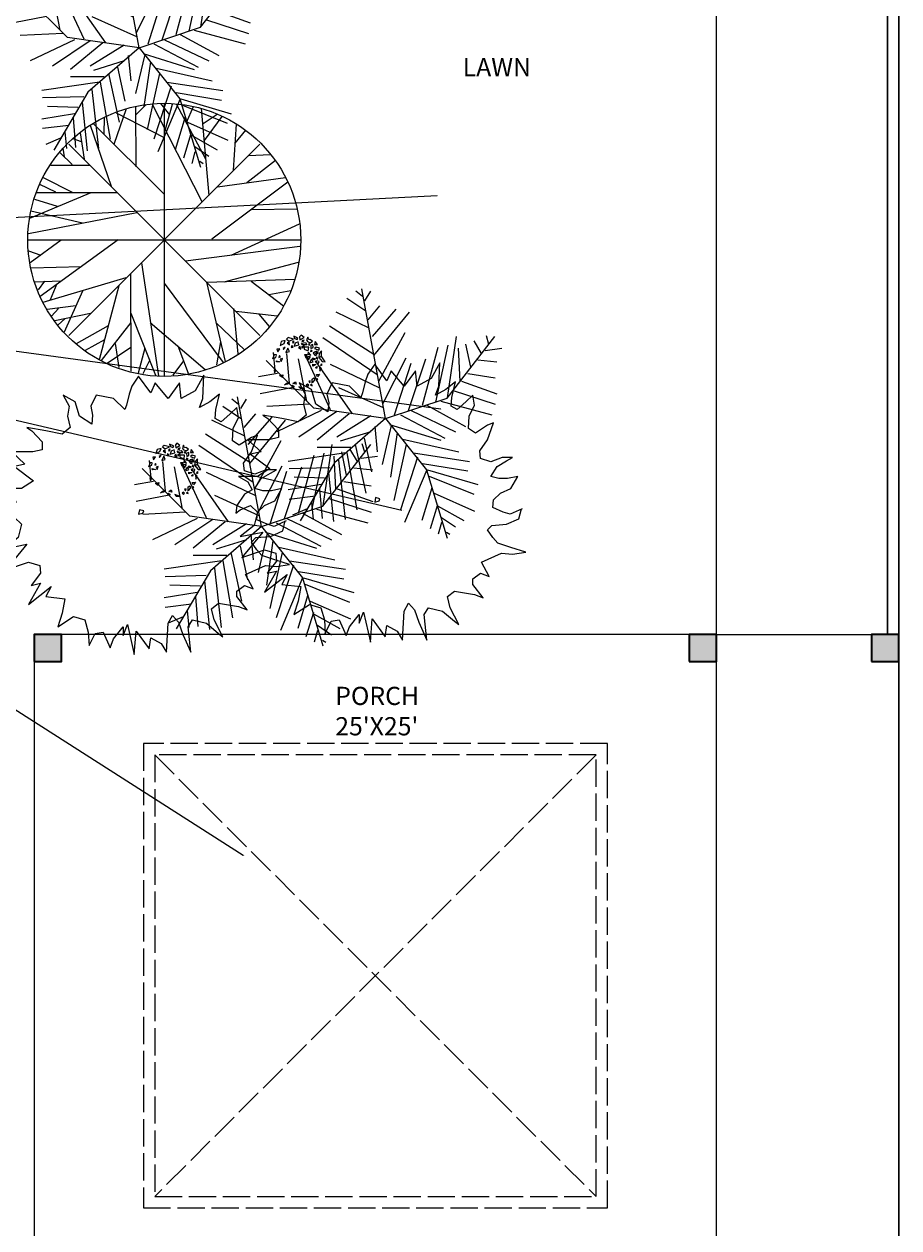
# Model space of a CAD drawing. Units: inches. Extents: x 2330 to 3943, y 1763 to 3461.
# Tile 23 of 40: x 3423 to 3808, y 2300 to 2829. Entities that reach past the tile are written whole.
import ezdxf

# ---------------------------------------------------------------- set-up
doc = ezdxf.new("R2010")
doc.units = ezdxf.units.IN
doc.linetypes.add('ACAD_ISO02W100', pattern=[15, 12, -3])
for name, color, linetype, lineweight in [('A-ANNO-DIMS', 2, 'Continuous', 18), ('A-ANNO-TEXT', 7, 'Continuous', 18), ('A-AREA-IDEN', 7, 'Continuous', 18), ('A-COLS', 7, 'Continuous', 35), ('A-FLOR', 7, 'Continuous', 25), ('A-ROOF-OVHD', 8, 'ACAD_ISO02W100', 18), ('C-PROP', 7, 'Continuous', 30), ('L-PLNT', 94, 'Continuous', 13)]:
    doc.layers.add(name, color=color, linetype=linetype, lineweight=lineweight)
doc.styles.get("Standard").update_dxf_attribs({"font": 'arial.ttf'})
doc.dimstyles.get("Standard").update_dxf_attribs({"dimtxt": 0.18, "dimasz": 0.18, "dimexe": 0.18, "dimexo": 0.0625, "dimgap": 0.09, "dimtad": 0, "dimtih": 1, "dimtoh": 1, "dimdec": 4, "dimzin": 0, "dimdsep": 46, "dimtxsty": 'Standard', "dimcen": 0.09, "dimadec": 0, "dimazin": 0, "dimtfac": 1, "dimtdec": 4, "dimtofl": 0, "dimtmove": 0, "dimatfit": 3, "dimfxl": 1, "dimtolj": 1, "dimtzin": 0, "dimarcsym": 0})

# ---------------------------------------------------------------- blocks, each defined once
blk = doc.blocks.new('*U12')
for p, q in [((-10.186, 53.64), (-13.084, 55.962)), ((0, 0), (-10.5, 57)), ((-9.099, 51.782), (-6.563, 55.962)), ((-8.737, 47.138), (-17.069, 52.711)), ((-7.65, 43.423), (-2.578, 49.46)), ((-5.839, 35.992), (4.667, 48.067)), ((-7.288, 39.707), (-21.778, 46.673)), ((-5.114, 27.632), (10.463, 46.673)), ((-5.114, 28.097), (-24.676, 40.636)), ((-2.941, 16.486), (8.652, 37.85)), ((-3.665, 19.273), (-27.574, 35.527)), ((22.055, 7.198), (27.489, 32.277)), ((27, 9), (48, 36)), ((27.127, 9.056), (31.112, 35.992)), ((35.096, 32.741), (37.27, 22.524)), ((38.719, 34.134), (41.979, 28.561)), ((44.153, 36.456), (45.239, 32.741)), ((-48.585, 21.131), (-49.309, 29.026)), ((-43.513, 28.561), (-42.427, 15.558)), ((-35.544, 28.097), (-24.314, 3.947)), ((-1.129, 6.734), (9.014, 26.704)), ((16.259, 5.805), (23.142, 31.348)), ((31.836, 30.883), (32.561, 16.486)), ((43.791, 29.954), (51.036, 30.883)), ((-31.5, 4.5), (-52.5, 25.5)), ((-38.442, 26.239), (-34.819, 7.663)), ((-14.533, 2.09), (-30.834, 25.31)), ((-24.314, 23.917), (-2.941, 13.7)), ((3.942, 1.625), (11.187, 24.381)), ((10.101, 3.483), (17.708, 26.239)), ((40.53, 25.775), (48.862, 24.846)), ((-47.498, 19.737), (-55.83, 18.344)), ((33.285, 16.486), (48.862, 10.913)), ((36.183, 19.737), (48.137, 17.88)), ((-40.615, 13.7), (-55.105, 10.913)), ((-20.691, 13.7), (-1.129, 4.876)), ((29.662, 12.307), (48.137, 6.269)), ((-33.37, 6.269), (-52.207, 5.34)), ((0, 0), (27, 9)), ((18.07, 5.805), (35.096, -3.483)), ((24.229, 7.663), (46.688, 1.625)), ((-28.299, 3.483), (-47.86, -5.805)), ((-21.416, 3.018), (-38.079, -8.128)), ((0, 0), (-31.5, 4.5)), ((-15.982, 2.09), (-30.11, -9.521)), ((0, 0), (-22.5, -19.5)), ((-6.563, 1.161), (-21.416, -8.128)), ((0, 0), (18, -22.5)), ((6.478, 1.625), (26.04, -8.592)), ((11.187, 3.483), (30.749, -5.805)), ((-4.752, -3.483), (-3.665, -14.629)), ((2.493, -3.019), (-1.491, -20.202)), ((1.769, -2.555), (24.229, -9.521)), ((-6.563, -5.805), (-19.967, -9.985)), ((-9.461, -8.592), (-6.201, -23.453)), ((5.029, -6.27), (2.131, -25.775)), ((7.565, -9.056), (32.198, -14.629)), ((-17.431, -15.094), (-42.789, -18.809)), ((-15.257, -12.772), (-30.11, -12.772)), ((-17.069, -15.094), (-12.721, -40.172)), ((-13.446, -11.378), (-8.737, -32.741)), ((9.014, -11.378), (3.58, -35.992)), ((12.274, -15.094), (36.907, -18.809)), ((-22.5, -19.5), (-37.5, -45)), ((-20.691, -18.345), (-17.793, -44.352)), ((14.085, -16.951), (6.478, -40.172)), ((16.259, -19.738), (36.183, -22.989)), ((-24.314, -21.596), (-42.427, -22.06)), ((-26.849, -26.24), (-40.253, -25.775)), ((-25.038, -23.918), (-22.865, -45.281)), ((18.07, -22.524), (8.289, -45.745)), ((18, -22.5), (27, -52.5)), ((18.433, -22.524), (40.53, -29.026)), ((19.157, -25.311), (38.719, -33.206)), ((-28.299, -29.026), (-42.789, -31.348)), ((-29.023, -30.884), (-27.936, -43.887)), ((20.244, -30.419), (15.897, -44.816)), ((-30.834, -34.135), (-42.427, -35.528)), ((-32.646, -36.921), (-31.921, -44.352)), ((21.331, -32.741), (39.081, -40.636)), ((-34.457, -39.708), (-40.978, -42.494)), ((22.78, -37.85), (19.519, -48.532)), ((22.78, -38.314), (34.372, -44.816)), ((24.591, -45.745), (23.142, -50.854)), ((24.591, -43.423), (30.749, -47.603)), ((26.764, -49.925), (28.213, -50.854))]:
    blk.add_line(p, q)
blk = doc.blocks.new('*U14')
for p, q in [((-12.5388, 54.9406), (-7.9613, 59.4546)), ((-12.3627, 32.1443), (-12.5388, 58.7776)), ((-5.3205, 59.6806), (16.5105, 16.7963)), ((2.426, 54.9406), (-1.4472, 59.9056)), ((0, 59.9996), (0, -60)), ((0.4894, 48.6208), (3.6584, 59.6806)), ((18.2711, 35.5298), (5.419, 59.6806)), ((9.8203, 51.5549), (12.8133, 58.5516)), ((-26.4472, 46.5894), (-26.2712, 53.8116)), ((-22.0458, 42.0753), (-16.5881, 57.6486)), ((-21.1656, 55.8436), (-0.0388, 45.0094)), ((19.6795, 19.5047), (16.3344, 57.6486)), ((17.0387, 51.1035), (23.2006, 55.1666)), ((17.7429, 43.6552), (25.4894, 54.2636)), ((-32.6092, 50.4264), (-23.2782, 23.5674)), ((-31.2008, 51.1035), (-0.2149, 20.1818)), ((31.6513, 50.8778), (30.2429, 30.5643)), ((31.1232, 42.5267), (35.8767, 48.1693)), ((-40.1797, 44.558), (-36.4825, 43.2038)), ((-37.0107, 47.0408), (-35.25, 35.5298)), ((-45.8134, 38.2383), (-40.5318, 33.0471)), ((-43.8768, 36.4326), (-44.405, 40.2696)), ((42, 42), (-42, -42)), ((42, -42), (-42, 42)), ((37.1091, 37.1098), (46.6161, 37.5612)), ((-49.8627, 32.8214), (-32.7853, 32.8214)), ((36.2288, 25.1474), (48.9049, 35.0784)), ((-53.2078, 27.4044), (-40.1797, 20.859)), ((23.3767, 23.3417), (53.3063, 27.4044)), ((-54.7923, 24.4702), (-47.75, 21.0847)), ((54.3626, 25.3731), (20.9119, 0.3198)), ((-32.2571, 20.6333), (-59.1937, 9.348)), ((-57.081, 17.9248), (-47.0458, 14.7649)), ((-56.0247, 20.859), (-20.8134, 20.859)), ((-59.7219, 2.8025), (-12.0106, 12.0565)), ((-58.6656, 12.7336), (-35.9543, 7.5424)), ((38.5175, 13.4107), (58.2359, 13.6364)), ((29.3626, -6.6771), (59.4682, 7.091)), ((-54.6162, -24.7335), (-20.2853, 0.0941)), ((-60, 0), (60, 0)), ((-59.7219, -4.8714), (-54.2641, -6.6771)), ((-45.2853, -0.1316), (-59.0177, -10.0627)), ((9.2922, -9.1598), (59.6443, -2.8401)), ((-10.074, -10.0627), (-2.5036, -59.7178)), ((26.3697, -18.4138), (58.9401, -9.8369)), ((-58.4895, -12.3197), (-36.4825, -11.6426)), ((-14.8275, -15.0282), (-14.6515, -57.6865)), ((-57.081, -18.4138), (-45.2853, -17.9624)), ((-52.6797, -18.188), (-55.4966, -22.0251)), ((-53.2078, -27.442), (-16.7641, -16.6081)), ((-47.2219, -19.3166), (-50.2148, -26.3135)), ((-19.9331, -20.2194), (-28.5599, -52.721)), ((-0.0388, -19.0909), (25.8415, -53.8495)), ((18.6232, -18.6394), (26.7218, -53.3981)), ((18.7992, -18.6394), (57.3556, -17.2853)), ((38.1654, -18.188), (52.426, -29.0219)), ((-35.9543, -22.4765), (-44.0529, -40.5329)), ((45.9119, -24.0564), (55.595, -22.2508)), ((-38.9472, -29.0219), (-51.4472, -30.6018)), ((-46.5177, -30.1504), (-49.5106, -33.536)), ((30.419, -30.1504), (32.3556, -50.0125)), ((31.4753, -31.279), (49.6091, -33.3103)), ((-32.4331, -32.4075), (-48.1021, -35.5674)), ((-43.7008, -34.6645), (-46.6937, -37.373)), ((-14.6515, -36.2445), (-27.6797, -52.9467)), ((-14.6515, -32.1818), (-3.912, -59.4922)), ((-6.2008, -36.2445), (17.919, -57.0094)), ((22.8485, -36.4702), (35.3485, -48.4326)), ((41.5105, -32.6332), (46.088, -38.0501)), ((-24.6867, -37.8244), (-38.7712, -45.7241)), ((-26.2712, -43.9185), (-34.7219, -48.6583)), ((-14.6515, -47.3041), (-25.0388, -54.3009)), ((-21.5177, -45.4984), (-19.9331, -56.1065)), ((-8.4895, -47.5298), (-11.4825, -58.5893)), ((5.9471, -46.6269), (10.5246, -58.5893)), ((24.7852, -44.8213), (23.0246, -54.978)), ((-6.3768, -52.721), (-9.3698, -58.815)), ((8.4119, -53.1724), (3.8344, -59.4922))]:
    blk.add_line(p, q)
blk.add_circle((0, 0), 60)
blk = doc.blocks.new('*U15')
for points in [[(0, 60.64), (-3.051, 56.238), (-4.196, 52.815), (-5.34, 47.925), (-6.103, 45.969), (-11.062, 50.859), (-18.691, 52.326), (-20.98, 47.436), (-20.217, 43.524), (-20.598, 39.611), (-25.939, 43.035), (-27.846, 49.392), (-33.186, 52.326), (-30.516, 47.436), (-31.279, 43.035), (-30.135, 38.144), (-33.568, 35.21), (-40.815, 36.677), (-49.208, 38.144), (-46.919, 36.677), (-42.341, 31.787), (-42.341, 28.364), (-46.537, 27.386), (-55.692, 27.386), (-49.97, 22.006), (-54.548, 21.028), (-46.156, 14.671), (-51.496, 11.248), (-59.888, 11.248), (-55.692, 8.803), (-53.785, 5.38), (-57.218, 3.423), (-60.651, -1.467), (-61.033, -4.89), (-59.125, -3.423), (-54.548, -1.467), (-51.496, -4.401), (-53.022, -10.269), (-59.125, -15.16), (-49.208, -13.204), (-58.362, -24.451), (-48.445, -21.028), (-43.486, -22.495), (-43.104, -25.918), (-47.3, -31.298), (-43.104, -30.32), (-48.445, -39.611), (-38.527, -31.787), (-40.815, -36.188), (-32.423, -37.166), (-33.568, -43.523), (-35.475, -49.392), (-28.609, -44.99), (-23.65, -46.457), (-22.124, -51.837), (-21.743, -57.705), (-19.073, -52.326), (-15.639, -51.837), (-12.588, -58.683), (-11.062, -54.771), (-6.866, -49.392), (-6.866, -53.304), (-4.959, -48.414), (-1.907, -61.617), (-1.144, -51.348), (4.578, -59.172), (5.341, -54.282), (9.918, -56.727), (12.207, -60.639), (12.97, -47.925), (14.877, -44.501), (17.547, -47.436), (19.455, -52.815), (22.888, -60.639), (21.743, -49.392), (23.65, -46.457), (29.754, -47.925), (35.094, -52.326), (37.001, -53.793), (33.187, -46.457), (32.042, -41.567), (35.094, -39.122), (43.868, -40.589), (47.682, -42.056), (43.105, -36.188), (43.105, -33.743), (46.538, -31.298), (50.352, -32.765), (46.919, -26.407), (55.693, -22.495), (60.652, -22.984), (66.374, -22.006), (59.889, -20.05), (54.167, -18.094), (51.878, -15.649), (49.589, -12.225), (51.497, -10.269), (57.981, -9.78), (63.322, -7.335), (64.466, -2.934)], [(64.848, -2.934), (59.507, -5.379), (56.456, -4.401), (51.878, -2.445), (52.26, 0.978), (55.311, 3.912), (59.889, 5.869), (62.94, 11.248), (58.363, 10.27), (54.548, 10.27), (51.115, 11.248), (53.785, 15.649), (57.981, 18.094), (60.652, 19.561), (56.074, 19.561), (51.115, 17.605), (46.538, 19.072), (46.156, 22.496), (49.589, 27.386), (52.26, 34.721), (49.589, 33.743), (44.249, 30.32), (41.197, 32.276), (41.579, 37.655), (43.868, 42.546), (43.105, 46.947), (40.053, 44.013), (36.238, 40.589), (33.568, 42.057), (33.95, 45.969), (35.476, 52.815), (31.28, 49.392), (26.702, 46.947), (28.228, 50.859), (28.609, 61.129), (24.795, 54.282), (18.692, 50.859), (17.929, 57.706), (12.97, 50.859), (7.248, 57.706), (5.341, 53.304), (0, 60.64)]]:
    blk.add_lwpolyline(points)
blk.add_lwpolyline([(0.382, 1.956), (0, 0), (1.907, 0.489), (2.289, 1.467)], close=True)
blk = doc.blocks.new('*U13')
for points in [[(-4.43, 11.05), (-5.18, 10.36), (-3.96, 9.49), (-2.07, 10.36)], [(-2, 11.66), (-1.6, 10.62), (-0.52, 10.1), (-0.18, 10.62), (-0.79, 10.96)], [(1.24, 12), (0.56, 11.31), (0.76, 10.01), (2.52, 11.05)], [(4.14, 11.14), (3.6, 10.01), (4, 9.23), (5.22, 8.71), (6.3, 9.41), (5.08, 10.19), (4.61, 10.01)], [(-8.14, 6.03), (-9.36, 5.95), (-9.02, 4.73)], [(-5.78, 9.75), (-7.54, 9.23), (-8.01, 7.5), (-6.26, 8.45)], [(-5.78, 6.81), (-6.66, 6.21), (-6.52, 5.69)], [(-4.57, 6.38), (-5.45, 4.47), (-3.89, 4.82)], [(-4.84, 8.63), (-3.83, 7.85), (-4.03, 8.97)], [(-2.88, 7.5), (-3.15, 6.64), (-2.27, 6.72)], [(-1.94, 9.49), (-2.48, 8.97), (-2.27, 8.54), (-1.8, 9.06)], [(0.02, 9.06), (-1.33, 8.54), (-1.73, 7.16), (0.29, 7.76)], [(0.76, 7.16), (0.09, 6.46), (1.1, 5.95)], [(1.37, 8.54), (3.13, 8.8), (3.8, 7.85), (1.91, 7.76)], [(2.59, 9.93), (1.84, 9.75), (1.64, 9.23), (2.32, 9.41)], [(1.71, 6.29), (1.71, 7.07), (2.65, 7.5), (2.11, 6.9)], [(2.52, 6.81), (2.52, 5.86), (4.41, 5.17), (4.61, 6.72)], [(4.61, 8.28), (4.54, 7.76), (4.95, 7.59), (4.95, 8.28)], [(5.49, 5.51), (5.42, 4.82), (6.16, 5.08)], [(6.43, 7.94), (5.49, 7.68), (5.56, 6.21), (6.5, 6.64)], [(7.45, 9.32), (7.11, 7.94), (8.52, 7.94)], [(7.85, 6.81), (7.18, 6.21), (9, 5.51), (9.33, 6.38)], [(-11.32, 1.79), (-9.83, 2.31), (-9.63, 3.44), (-10.44, 3.52)], [(-8.21, 0.41), (-9.43, 0.32), (-9.83, 0.84)], [(-8.21, 3.09), (-8.48, 2.31), (-7.87, 2.57)], [(-7, 1.79), (-7.94, 1.53), (-7.47, 0.49)], [(3.53, 1.88), (2.86, 3.52), (3.8, 3.52)], [(4.41, 4.56), (4.27, 3.7), (5.49, 3.26)], [(4.27, 2.74), (5.29, 2.66), (4.41, 1.27)], [(5.83, 1.53), (5.02, 0.41), (5.49, -0.02), (6.5, 0.41)], [(7.51, 1.71), (6.91, 1.27), (6.23, 2.14)], [(8.12, 4.99), (7.11, 4.65), (6.5, 4.13), (7.38, 3.09), (8.12, 3.52), (7.65, 3.87)], [(8.12, 0.75), (7.51, 0.15), (8.93, -0.28), (9.13, 0.49)], [(8.19, 2.57), (7.92, 2.05), (8.66, 1.53)], [(8.73, 4.73), (8.19, 4.56), (8.39, 3.87), (8.59, 4.04)], [(10.28, 5.17), (9.2, 4.04), (9, 2.31), (10.48, 0.49), (11.76, 0.41), (10.35, 2.48), (9.33, 2.4), (10.28, 2.83)], [(-10.03, -2.71), (-10.64, -3.31), (-10.44, -4.44), (-9.9, -3.49)], [(7.78, -0.8), (6.43, -1.5), (6.43, -0.72)], [(8.32, -1.75), (7.98, -2.53), (7.58, -2.1)], [(9.33, -5.13), (8.46, -6.25), (7.98, -5.22)], [(9.33, -1.75), (9.54, -3.74), (10.14, -2.53)], [(10.08, -0.63), (9.74, -1.32), (10.48, -0.89)], [(-8.28, -5.73), (-6.79, -5.3), (-7, -6.51)], [(-4.84, -8.85), (-4.43, -9.45), (-5.99, -9.8)], [(-2.54, -10.06), (-3.02, -10.23), (-1.8, -10.67)], [(-2.34, -9.2), (-1.26, -8.5), (-0.99, -9.54)], [(4.07, -9.45), (3.53, -9.97), (4.07, -10.58), (4.61, -9.89)], [(5.29, -7.98), (4.61, -8.16), (5.02, -8.94)], [(6.03, -9.45), (5.42, -9.97), (6.16, -10.15)], [(6.1, -8.94), (6.16, -7.21), (6.91, -6.69), (7.24, -7.38)], [(8.05, -8.07), (8.59, -7.12), (7.92, -7.55)], [(0.22, -10.58), (0.83, -11.27), (2.59, -11.36)]]:
    blk.add_lwpolyline(points, close=True)
blk = doc.blocks.new('POST-PORCH-12IN')
h = blk.add_hatch(color=256)
h.dxf.hatch_style = 1
h.paths.add_polyline_path([(12, 12), (0, 12), (0, 0), (12, 0)])
blk.add_lwpolyline([(0, 0), (12, 0), (12, 12), (0, 12)], close=True)
blk = doc.blocks.new('*D67')
at = {"layer": 'A-ANNO-DIMS', "color": 0, "lineweight": -2, "transparency": 16777216}
for p, q in [((3727.52, 2560.76), (3727.52, 3461.3)), ((3727.7, 3461.12), (3767.19, 3461.12)), ((3807.48, 3461.12), (3767.98, 3461.12)), ((3807.66, 2560.76), (3807.66, 3461.3))]:
    blk.add_line(p, q, dxfattribs=at)
at = {"layer": 'A-ANNO-DIMS', "color": 0, "transparency": 16777216}
for points in [[(3727.7, 3461.15), (3727.7, 3461.09), (3727.52, 3461.12)], [(3807.48, 3461.15), (3807.48, 3461.09), (3807.66, 3461.12)]]:
    blk.add_solid(points, dxfattribs=at)
at = {"layer": 'Defpoints', "color": 0, "transparency": 16777216}
for p in [(3807.66, 3461.12), (3727.52, 2560.7), (3807.66, 2560.7)]:
    blk.add_point(p, dxfattribs=at)
at = {"layer": 'A-ANNO-DIMS', "color": 0, "transparency": 16777216, "insert": (3767.59, 3461.12), "char_height": 0.18, "attachment_point": 5}
blk.add_mtext('\\A1;80.14', dxfattribs=at)
blk = doc.blocks.new('*D95')
at = {"layer": 'A-ANNO-DIMS', "color": 0, "lineweight": -2, "transparency": 16777216}
for p, q in [((3105.6, 2727.69), (3105.78, 2727.69)), ((3105.69, 2727.6), (3105.69, 2727.78)), ((3606.31, 2659.69), (3418.76, 2685.16))]:
    blk.add_line(p, q, dxfattribs=at)
at = {"layer": 'A-ANNO-DIMS', "color": 0, "transparency": 16777216}
blk.add_solid([(3418.76, 2685.19), (3418.75, 2685.14), (3418.58, 2685.19)], dxfattribs=at)
at = {"layer": 'Defpoints', "color": 0, "transparency": 16777216}
for p in [(3105.69, 2727.69), (3418.58, 2685.19)]:
    blk.add_point(p, dxfattribs=at)
at = {"layer": 'A-ANNO-DIMS', "color": 0, "transparency": 16777216, "insert": (3606.86, 2659.69), "char_height": 0.18, "attachment_point": 5}
blk.add_mtext('\\A1;R315.76', dxfattribs=at)
blk = doc.blocks.new('*D96')
at = {"layer": 'A-ANNO-DIMS', "color": 0, "lineweight": -2, "transparency": 16777216}
for p, q in [((3604.65, 2753.34), (3417.72, 2743.73)), ((3105.6, 2727.69), (3105.78, 2727.69)), ((3105.69, 2727.6), (3105.69, 2727.78))]:
    blk.add_line(p, q, dxfattribs=at)
at = {"layer": 'A-ANNO-DIMS', "color": 0, "transparency": 16777216}
blk.add_solid([(3417.72, 2743.76), (3417.72, 2743.7), (3417.54, 2743.72)], dxfattribs=at)
at = {"layer": 'Defpoints', "color": 0, "transparency": 16777216}
for p in [(3417.54, 2743.72), (3105.69, 2727.69)]:
    blk.add_point(p, dxfattribs=at)
at = {"layer": 'A-ANNO-DIMS', "color": 0, "transparency": 16777216, "insert": (3605.39, 2753.34), "char_height": 0.18, "attachment_point": 5}
blk.add_mtext('\\A1;2X R312.26', dxfattribs=at)
blk = doc.blocks.new('*D97')
at = {"layer": 'A-ANNO-DIMS', "color": 0, "lineweight": -2, "transparency": 16777216}
for p, q in [((3105.6, 2727.69), (3105.78, 2727.69)), ((3105.69, 2727.6), (3105.69, 2727.78)), ((3589.17, 2615.07), (3408.04, 2657.26))]:
    blk.add_line(p, q, dxfattribs=at)
at = {"layer": 'A-ANNO-DIMS', "color": 0, "transparency": 16777216}
blk.add_solid([(3408.05, 2657.29), (3408.03, 2657.23), (3407.86, 2657.3)], dxfattribs=at)
at = {"layer": 'Defpoints', "color": 0, "transparency": 16777216}
for p in [(3105.69, 2727.69), (3407.86, 2657.3)]:
    blk.add_point(p, dxfattribs=at)
at = {"layer": 'A-ANNO-DIMS', "color": 0, "transparency": 16777216, "insert": (3589.91, 2615.07), "char_height": 0.18, "attachment_point": 5}
blk.add_mtext('\\A1;2X R310.26', dxfattribs=at)
blk = doc.blocks.new('*D98')
at = {"layer": 'A-ANNO-DIMS', "color": 0, "lineweight": -2, "transparency": 16777216}
for p, q in [((3105.6, 2727.69), (3105.78, 2727.69)), ((3105.69, 2727.6), (3105.69, 2727.78)), ((3519.33, 2463.49), (3364.37, 2562.47)), ((3519.51, 2463.49), (3519.33, 2463.49))]:
    blk.add_line(p, q, dxfattribs=at)
at = {"layer": 'A-ANNO-DIMS', "color": 0, "transparency": 16777216}
blk.add_solid([(3364.39, 2562.49), (3364.35, 2562.44), (3364.22, 2562.56)], dxfattribs=at)
at = {"layer": 'Defpoints', "color": 0, "transparency": 16777216}
for p in [(3105.69, 2727.69), (3364.22, 2562.56)]:
    blk.add_point(p, dxfattribs=at)
at = {"layer": 'A-ANNO-DIMS', "color": 0, "transparency": 16777216, "insert": (3520.26, 2463.49), "char_height": 0.18, "attachment_point": 5}
blk.add_mtext('\\A1;3X R306.76', dxfattribs=at)

msp = doc.modelspace()

# ---------------------------------------------------------------- linework, layer by layer
at = {"layer": 'A-FLOR'}
msp.add_line((3727.5159, 2560.7019), (3807.6605, 2560.7019), dxfattribs=at)
msp.add_lwpolyline([(3427.5159, 2260.7019), (3727.5159, 2260.7019), (3727.5159, 2560.7019), (3427.5159, 2560.7019)], close=True, dxfattribs=at)
at = {"layer": 'A-ROOF-OVHD'}
for p, q in [((3674.5159, 2507.7019), (3480.5159, 2313.7019)), ((3480.5159, 2507.7019), (3674.5159, 2313.7019))]:
    msp.add_line(p, q, dxfattribs=at)
for points in [[(3475.5159, 2308.7019), (3679.5159, 2308.7019), (3679.5159, 2512.7019), (3475.5159, 2512.7019)], [(3480.5159, 2313.7019), (3674.5159, 2313.7019), (3674.5159, 2507.7019), (3480.5159, 2507.7019)]]:
    msp.add_lwpolyline(points, close=True, dxfattribs=at)
at = {"layer": 'C-PROP'}
for p, q in [((3802.6605, 3205.6524), (3802.6605, 2560.7019)), ((3807.6605, 3210.6524), (3807.6605, 1974.6524))]:
    msp.add_line(p, q, dxfattribs=at)

# ---------------------------------------------------------------- block references
at = {"layer": 'A-COLS'}
for p in [(3427.5159, 2548.7019), (3715.5159, 2548.7019), (3795.6605, 2548.7019)]:
    msp.add_blockref('POST-PORCH-12IN', p, dxfattribs=at)
at = {"layer": 'L-PLNT'}
for name, p in [('*U12', (3473.6244, 2818.4657)), ('*U14', (3484.72, 2734.0264)), ('*U12', (3582.0198, 2655.5229)), ('*U13', (3543.6201, 2680.0961)), ('*U15', (3577.2128, 2618.8419)), ('*U15', (3473.4568, 2613.4629)), ('*U12', (3527.4718, 2608.0869)), ('*U13', (3489.0721, 2632.6601))]:
    msp.add_blockref(name, p, dxfattribs=at)

# ---------------------------------------------------------------- texts
at = {"layer": 'A-ANNO-TEXT', "insert": (3615.8887, 2813.8967), "char_height": 8, "attachment_point": 1}
msp.add_mtext_dynamic_manual_height_columns('LAWN', width=151.739694, gutter_width=12.5, heights=[0], dxfattribs=at)
at = {"layer": 'A-AREA-IDEN', "insert": (3559.8674, 2537.6491), "char_height": 8, "attachment_point": 1}
msp.add_mtext_dynamic_manual_height_columns("PORCH\\P25'X25'", width=125.525054, gutter_width=12.5, heights=[0], dxfattribs=at)

# ---------------------------------------------------------------- dimensions: what is measured, and where the dimension line sits
at = {"layer": 'A-ANNO-DIMS'}
dim = msp.add_linear_dim(base=(3807.6605, 3461.1231), p1=(3727.5159, 2560.7019), p2=(3807.6605, 2560.7019), dimstyle='Standard', override={"dimdec": 2, "dimlfac": 1, "dimrnd": 0, "dimzin": 0, "dimdsep": 46, "dimlunit": 2}, dxfattribs=at)
dim.commit()
dim.dimension.update_dxf_attribs({"geometry": '*D67', "text_midpoint": (3767.5882, 3461.1231)})
for mpoint, text, picture, middle in [((3417.5409, 2743.723), '2X <>', '*D96', (3604.6494, 2753.3446)), ((3407.8638, 2657.302), '2X <>', '*D97', (3589.166, 2615.0711)), ((3364.219, 2562.563), '3X <>', '*D98', (3520.2574, 2463.4886))]:
    dim = msp.add_radius_dim(center=(3105.6935, 2727.6869), mpoint=mpoint, text=text, dimstyle='Standard', override={"dimdec": 2, "dimlfac": 1, "dimrnd": 0, "dimzin": 0, "dimdsep": 46, "dimlunit": 2}, dxfattribs=at)
    dim.commit()
    dim.dimension.update_dxf_attribs({"geometry": picture, "text_midpoint": middle, "dimtype": 164})
dim = msp.add_radius_dim(center=(3105.6935, 2727.6869), mpoint=(3418.58, 2685.189), dimstyle='Standard', override={"dimdec": 2, "dimlfac": 1, "dimrnd": 0, "dimzin": 0, "dimdsep": 46, "dimlunit": 2}, dxfattribs=at)
dim.commit()
dim.dimension.update_dxf_attribs({"geometry": '*D95', "text_midpoint": (3606.3119, 2659.6902), "dimtype": 164})

doc.saveas('drawing.dxf')
